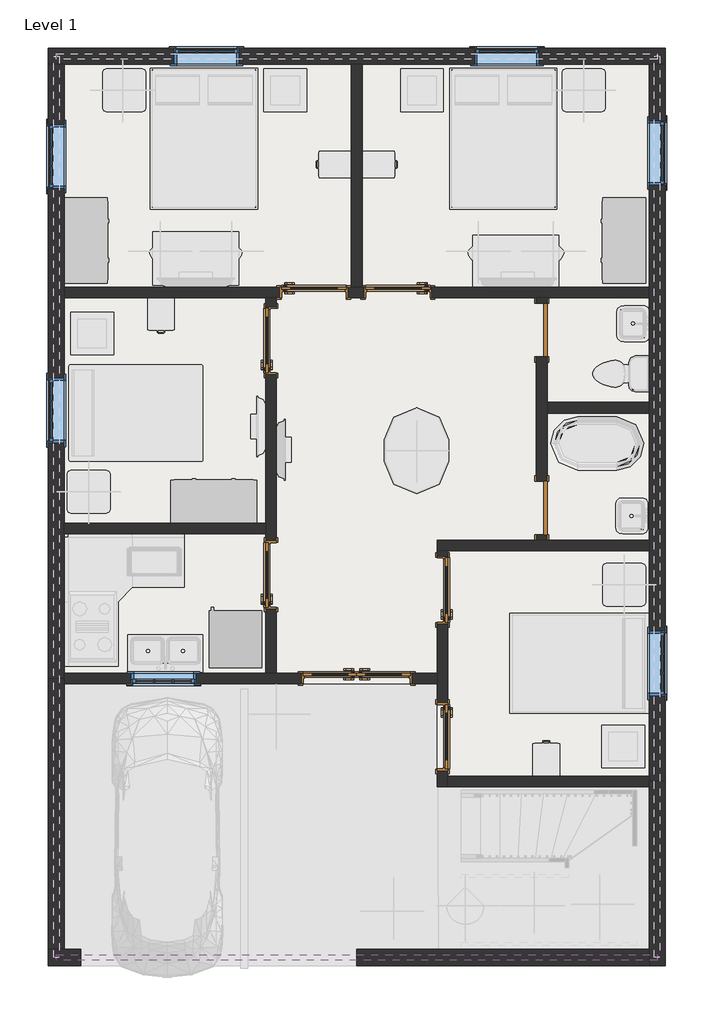
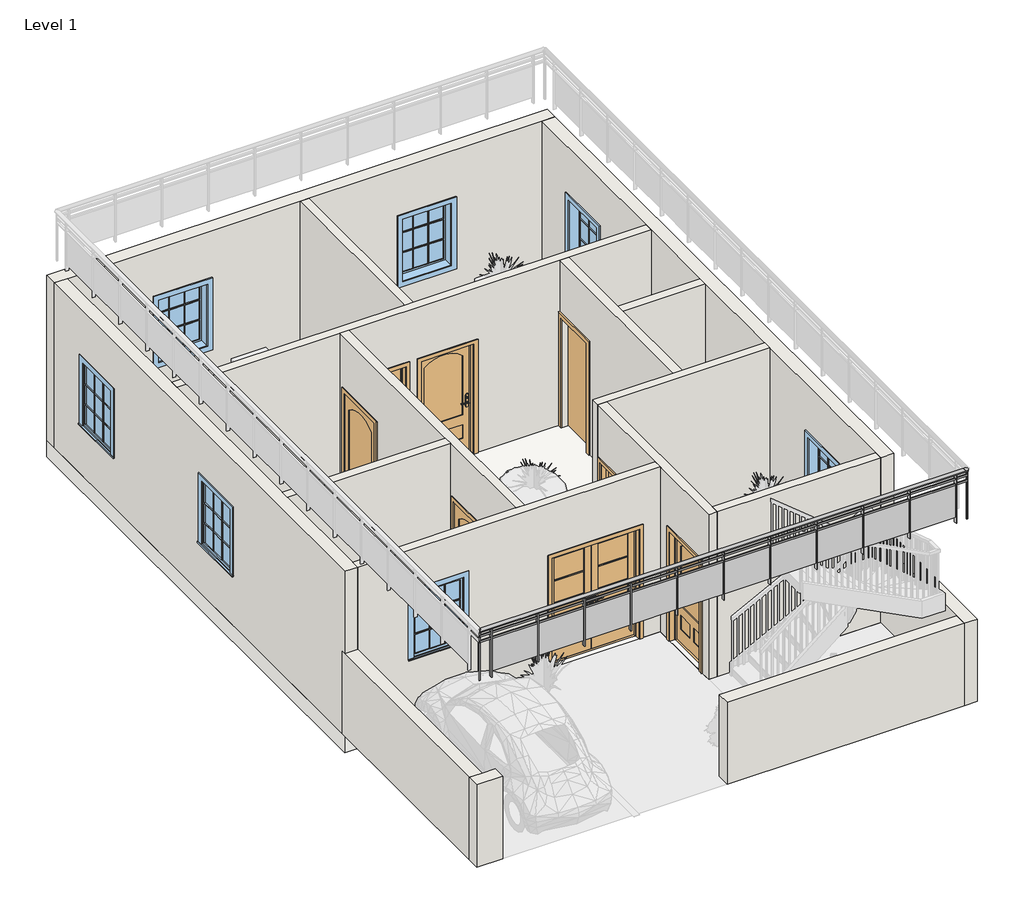
# One storey, part 1 of 4: 17 walls, 9 doors, 7 windows, 1 railing, 1 slab.
"""IFC4 building model written with IfcOpenShell, lengths in millimetres."""

from ifc_helpers import new_model, si_unit, point, frame, origin, origin_with_axes, place, context, project, spatial, polyline, ellipse_curve, trimmed, outline, extrude, faceted_brep, transform, mapped, element, save
from ifc_brep_helpers import plane_surface, extruded_surface, advanced_brep
from components import door_5d363d20, door_808aeb8e, door_94998e6c, door_255cab33, door_059fdd7e, window_b7d400b3, window_5c190c7e

model = new_model("IFC4")

# Units and contexts
model_context = context("Model", 3, world=origin())
ifc_project = project(units=[si_unit("LENGTHUNIT", "METRE", prefix="MILLI")], contexts=[model_context])

# Site, building, storey
site = spatial("IfcSite", under=ifc_project)
building = spatial("IfcBuilding", under=site)
storey = spatial("IfcBuildingStorey", under=building, Name="Level 1", Elevation=0.0)

# Doors
placement = place(None, origin())
door_shape = door_5d363d20(model_context)
element("IfcDoor", 1, ObjectType="36\" x 80\"", at=placement, inside=storey, context=model_context, shape_type="MappedRepresentation", body=[
    mapped(door_shape, transform((-9076.3505662, 9737.6395941, 0.0), x_axis=(-1.0, 0.0, 0.0), y_axis=(0.0, -1.0, 0.0), z_axis=(0.0, 0.0, 1.0))),
])
element("IfcDoor", 2, ObjectType="36\" x 80\"", at=placement, inside=storey, context=model_context, shape_type="MappedRepresentation", body=[
    mapped(door_shape, transform((-9689.1255662, 9048.6645941, 0.0), x_axis=(0.0, -1.0, 0.0), y_axis=(1.0, 0.0, 0.0), z_axis=(0.0, 0.0, 1.0))),
])
element("IfcDoor", 3, ObjectType="36\" x 80\"", at=placement, inside=storey, context=model_context, shape_type="MappedRepresentation", body=[
    mapped(door_shape, transform((-9689.1255662, 5721.2645941, 0.0), x_axis=(0.0, -1.0, 0.0), y_axis=(1.0, 0.0, 0.0), z_axis=(0.0, 0.0, 1.0))),
])
element("IfcDoor", 4, ObjectType="36\" x 80\"", at=placement, inside=storey, context=model_context, shape_type="MappedRepresentation", body=[
    mapped(door_shape, transform((-7244.3755662, 3422.5645941, 0.0), x_axis=(0.0, 1.0, 0.0), y_axis=(-1.0, 0.0, 0.0), z_axis=(0.0, 0.0, 1.0))),
])
door_2_shape = door_808aeb8e(model_context)
element("IfcDoor", 5, ObjectType="36\" x 80\"", at=placement, inside=storey, context=model_context, shape_type="MappedRepresentation", body=[
    mapped(door_2_shape, transform((-7882.5505662, 9737.6395941, 0.0), x_axis=(1.0, 0.0, 0.0), y_axis=(0.0, 1.0, 0.0), z_axis=(0.0, 0.0, 1.0))),
])
element("IfcDoor", 6, ObjectType="36\" x 80\"", at=placement, inside=storey, context=model_context, shape_type="MappedRepresentation", body=[
    mapped(door_2_shape, transform((-7244.3755662, 5505.3645941, 0.0), x_axis=(0.0, -1.0, 0.0), y_axis=(1.0, 0.0, 0.0), z_axis=(0.0, 0.0, 1.0))),
])
door_3_shape = door_94998e6c(model_context)
element("IfcDoor", 7, ObjectType="Door-Exterior-Double-Full Glass-Wood_Clad : 60\" x 80\"", at=placement, inside=storey, context=model_context, shape_type="MappedRepresentation", body=[
    mapped(door_3_shape, transform((-8466.7505662, 4251.2395941, 0.0), x_axis=(1.0, 0.0, 0.0), y_axis=(0.0, 1.0, 0.0), z_axis=(0.0, 0.0, 1.0))),
])
door_4_shape = door_255cab33(model_context)
element("IfcDoor", 8, ObjectType="Single-Flush : 30\" x 80\"", at=placement, inside=storey, context=model_context, shape_type="MappedRepresentation", body=[
    mapped(door_4_shape, transform((-5837.8505662, 9201.0645941, 0.0), x_axis=(0.0, 1.0, 0.0), y_axis=(-1.0, 0.0, 0.0), z_axis=(0.0, 0.0, 1.0))),
])
door_5_shape = door_059fdd7e(model_context)
element("IfcDoor", 9, ObjectType="Single-Flush : 30\" x 80\"", at=placement, inside=storey, context=model_context, shape_type="MappedRepresentation", body=[
    mapped(door_5_shape, transform((-5837.8505662, 6673.7645941, 0.0), x_axis=(0.0, -1.0, 0.0), y_axis=(1.0, 0.0, 0.0), z_axis=(0.0, 0.0, 1.0))),
])

# Railing
element("IfcRailing", 10, ObjectType="Glass Panel - Bottom Fill", at=placement, inside=storey, context=model_context, shape_type="SolidModel", body=[
    advanced_brep(
    [(-4199.5505662, 247.5645941, 4267.2), (-4199.5505662, 323.7645941, 4267.2), (-12733.9505662, 247.5645941, 4267.2), (-12733.9505662, 323.7645941, 4267.2)],
    [
        (0, 1, ellipse_curve(frame((-4199.5505662, 285.6645941, 4267.2), z_axis=(1.0, 0.0, 0.0), x_axis=(0.0, 1.0, 0.0)), 38.1, 28.575)),
        (1, 0, ellipse_curve(frame((-4199.5505662, 285.6645941, 4267.2), z_axis=(1.0, 0.0, 0.0), x_axis=(0.0, 1.0, 0.0)), 38.1, 28.575)),
        (2, 3, ellipse_curve(frame((-12733.9505662, 285.6645941, 4267.2), z_axis=(-1.0, 0.0, 0.0), x_axis=(0.0, 1.0, 0.0)), 38.1, 28.575)),
        (3, 2, ellipse_curve(frame((-12733.9505662, 285.6645941, 4267.2), z_axis=(-1.0, 0.0, 0.0), x_axis=(0.0, 1.0, 0.0)), 38.1, 28.575)),
        (0, 2),
        (3, 1),
    ],
    [
        plane_surface(frame((-4199.5505662, 285.6645941, 4267.2), z_axis=(1.0, 0.0, 0.0), x_axis=(0.0, -1.0, 0.0))),
        plane_surface(frame((-12733.9505662, 285.6645941, 4267.2), z_axis=(-1.0, 0.0, 0.0), x_axis=(0.0, -1.0, 0.0))),
        extruded_surface(trimmed(ellipse_curve(frame((-12733.9505662, 285.6645941, 4267.2), z_axis=(1.0, 0.0, 0.0), x_axis=(0.0, 1.0, 0.0)), 38.1, 28.575), [point((-12733.9505662, 247.5645941, 4267.2))], [point((-12733.9505662, 323.7645941, 4267.2))], True, "CARTESIAN"), (8534.4, 0.0, 0.0), 8534.4),
        extruded_surface(trimmed(ellipse_curve(frame((-12733.9505662, 285.6645941, 4267.2), z_axis=(1.0, 0.0, 0.0), x_axis=(0.0, 1.0, 0.0)), 38.1, 28.575), [point((-12733.9505662, 323.7645941, 4267.2))], [point((-12733.9505662, 247.5645941, 4267.2))], True, "CARTESIAN"), (8534.4, 0.0, 0.0), 8534.4),
    ],
    [
        (0, [[1, 2]]),
        (1, [[3, 4]]),
        (2, [[-1, 5, -4, 6]]),
        (3, [[-2, -6, -3, -5]]),
    ],
),
    extrude(outline(polyline([(-4199.5505662, 298.3645941), (-4199.5505662, 272.9645941), (-12733.9505662, 272.9645941), (-12733.9505662, 298.3645941), (-4199.5505662, 298.3645941)])), frame((0.0, 0.0, 4152.9), z_axis=(0.0, 0.0, 1.0), x_axis=(1.0, 0.0, 0.0)), (0.0, 0.0, 1.0), 25.4),
    extrude(outline(polyline([(-4199.5505662, 298.3645941), (-4199.5505662, 272.9645941), (-12733.9505662, 272.9645941), (-12733.9505662, 298.3645941), (-4199.5505662, 298.3645941)])), frame((0.0, 0.0, 4051.3), z_axis=(0.0, 0.0, 1.0), x_axis=(1.0, 0.0, 0.0)), (0.0, 0.0, 1.0), 25.4),
    extrude(outline(polyline([(-12524.4005662, 311.0645941), (-12524.4005662, 260.2645941), (-12537.1005662, 260.2645941), (-12537.1005662, 311.0645941), (-12524.4005662, 311.0645941)])), frame((0.0, 0.0, 3352.8), z_axis=(0.0, 0.0, 1.0), x_axis=(1.0, 0.0, 0.0)), (0.0, 0.0, 1.0), 885.6788223),
    extrude(outline(polyline([(-11717.9505662, 279.1294371), (-12530.7505662, 279.1294371), (-12530.7505662, 285.4794371), (-11717.9505662, 285.4794371), (-11717.9505662, 279.1294371)])), frame((0.0, 0.0, 3454.4), z_axis=(0.0, 0.0, 1.0), x_axis=(1.0, 0.0, 0.0)), (0.0, 0.0, 1.0), 596.9),
    extrude(outline(polyline([(-11711.6005662, 311.0645941), (-11711.6005662, 260.2645941), (-11724.3005662, 260.2645941), (-11724.3005662, 311.0645941), (-11711.6005662, 311.0645941)])), frame((0.0, 0.0, 3352.8), z_axis=(0.0, 0.0, 1.0), x_axis=(1.0, 0.0, 0.0)), (0.0, 0.0, 1.0), 885.6788223),
    extrude(outline(polyline([(-10905.1505662, 279.1294371), (-11717.9505662, 279.1294371), (-11717.9505662, 285.4794371), (-10905.1505662, 285.4794371), (-10905.1505662, 279.1294371)])), frame((0.0, 0.0, 3454.4), z_axis=(0.0, 0.0, 1.0), x_axis=(1.0, 0.0, 0.0)), (0.0, 0.0, 1.0), 596.9),
    extrude(outline(polyline([(-10898.8005662, 311.0645941), (-10898.8005662, 260.2645941), (-10911.5005662, 260.2645941), (-10911.5005662, 311.0645941), (-10898.8005662, 311.0645941)])), frame((0.0, 0.0, 3352.8), z_axis=(0.0, 0.0, 1.0), x_axis=(1.0, 0.0, 0.0)), (0.0, 0.0, 1.0), 885.6788223),
    extrude(outline(polyline([(-10092.3505662, 279.1294371), (-10905.1505662, 279.1294371), (-10905.1505662, 285.4794371), (-10092.3505662, 285.4794371), (-10092.3505662, 279.1294371)])), frame((0.0, 0.0, 3454.4), z_axis=(0.0, 0.0, 1.0), x_axis=(1.0, 0.0, 0.0)), (0.0, 0.0, 1.0), 596.9),
    extrude(outline(polyline([(-10086.0005662, 311.0645941), (-10086.0005662, 260.2645941), (-10098.7005662, 260.2645941), (-10098.7005662, 311.0645941), (-10086.0005662, 311.0645941)])), frame((0.0, 0.0, 3352.8), z_axis=(0.0, 0.0, 1.0), x_axis=(1.0, 0.0, 0.0)), (0.0, 0.0, 1.0), 885.6788223),
    extrude(outline(polyline([(-9279.5505662, 279.1294371), (-10092.3505662, 279.1294371), (-10092.3505662, 285.4794371), (-9279.5505662, 285.4794371), (-9279.5505662, 279.1294371)])), frame((0.0, 0.0, 3454.4), z_axis=(0.0, 0.0, 1.0), x_axis=(1.0, 0.0, 0.0)), (0.0, 0.0, 1.0), 596.9),
    extrude(outline(polyline([(-9273.2005662, 311.0645941), (-9273.2005662, 260.2645941), (-9285.9005662, 260.2645941), (-9285.9005662, 311.0645941), (-9273.2005662, 311.0645941)])), frame((0.0, 0.0, 3352.8), z_axis=(0.0, 0.0, 1.0), x_axis=(1.0, 0.0, 0.0)), (0.0, 0.0, 1.0), 885.6788223),
    extrude(outline(polyline([(-8466.7505662, 279.1294371), (-9279.5505662, 279.1294371), (-9279.5505662, 285.4794371), (-8466.7505662, 285.4794371), (-8466.7505662, 279.1294371)])), frame((0.0, 0.0, 3454.4), z_axis=(0.0, 0.0, 1.0), x_axis=(1.0, 0.0, 0.0)), (0.0, 0.0, 1.0), 596.9),
    extrude(outline(polyline([(-8460.4005662, 311.0645941), (-8460.4005662, 260.2645941), (-8473.1005662, 260.2645941), (-8473.1005662, 311.0645941), (-8460.4005662, 311.0645941)])), frame((0.0, 0.0, 3352.8), z_axis=(0.0, 0.0, 1.0), x_axis=(1.0, 0.0, 0.0)), (0.0, 0.0, 1.0), 885.6788223),
    extrude(outline(polyline([(-7653.9505662, 279.1294371), (-8466.7505662, 279.1294371), (-8466.7505662, 285.4794371), (-7653.9505662, 285.4794371), (-7653.9505662, 279.1294371)])), frame((0.0, 0.0, 3454.4), z_axis=(0.0, 0.0, 1.0), x_axis=(1.0, 0.0, 0.0)), (0.0, 0.0, 1.0), 596.9),
    extrude(outline(polyline([(-7647.6005662, 311.0645941), (-7647.6005662, 260.2645941), (-7660.3005662, 260.2645941), (-7660.3005662, 311.0645941), (-7647.6005662, 311.0645941)])), frame((0.0, 0.0, 3352.8), z_axis=(0.0, 0.0, 1.0), x_axis=(1.0, 0.0, 0.0)), (0.0, 0.0, 1.0), 885.6788223),
    extrude(outline(polyline([(-6841.1505662, 279.1294371), (-7653.9505662, 279.1294371), (-7653.9505662, 285.4794371), (-6841.1505662, 285.4794371), (-6841.1505662, 279.1294371)])), frame((0.0, 0.0, 3454.4), z_axis=(0.0, 0.0, 1.0), x_axis=(1.0, 0.0, 0.0)), (0.0, 0.0, 1.0), 596.9),
    extrude(outline(polyline([(-6834.8005662, 311.0645941), (-6834.8005662, 260.2645941), (-6847.5005662, 260.2645941), (-6847.5005662, 311.0645941), (-6834.8005662, 311.0645941)])), frame((0.0, 0.0, 3352.8), z_axis=(0.0, 0.0, 1.0), x_axis=(1.0, 0.0, 0.0)), (0.0, 0.0, 1.0), 885.6788223),
    extrude(outline(polyline([(-6028.3505662, 279.1294371), (-6841.1505662, 279.1294371), (-6841.1505662, 285.4794371), (-6028.3505662, 285.4794371), (-6028.3505662, 279.1294371)])), frame((0.0, 0.0, 3454.4), z_axis=(0.0, 0.0, 1.0), x_axis=(1.0, 0.0, 0.0)), (0.0, 0.0, 1.0), 596.9),
    extrude(outline(polyline([(-6022.0005662, 311.0645941), (-6022.0005662, 260.2645941), (-6034.7005662, 260.2645941), (-6034.7005662, 311.0645941), (-6022.0005662, 311.0645941)])), frame((0.0, 0.0, 3352.8), z_axis=(0.0, 0.0, 1.0), x_axis=(1.0, 0.0, 0.0)), (0.0, 0.0, 1.0), 885.6788223),
    extrude(outline(polyline([(-5215.5505662, 279.1294371), (-6028.3505662, 279.1294371), (-6028.3505662, 285.4794371), (-5215.5505662, 285.4794371), (-5215.5505662, 279.1294371)])), frame((0.0, 0.0, 3454.4), z_axis=(0.0, 0.0, 1.0), x_axis=(1.0, 0.0, 0.0)), (0.0, 0.0, 1.0), 596.9),
    extrude(outline(polyline([(-5209.2005662, 311.0645941), (-5209.2005662, 260.2645941), (-5221.9005662, 260.2645941), (-5221.9005662, 311.0645941), (-5209.2005662, 311.0645941)])), frame((0.0, 0.0, 3352.8), z_axis=(0.0, 0.0, 1.0), x_axis=(1.0, 0.0, 0.0)), (0.0, 0.0, 1.0), 885.6788223),
    extrude(outline(polyline([(-4402.7505662, 279.1294371), (-5215.5505662, 279.1294371), (-5215.5505662, 285.4794371), (-4402.7505662, 285.4794371), (-4402.7505662, 279.1294371)])), frame((0.0, 0.0, 3454.4), z_axis=(0.0, 0.0, 1.0), x_axis=(1.0, 0.0, 0.0)), (0.0, 0.0, 1.0), 596.9),
    extrude(outline(polyline([(-4396.4005662, 311.0645941), (-4396.4005662, 260.2645941), (-4409.1005662, 260.2645941), (-4409.1005662, 311.0645941), (-4396.4005662, 311.0645941)])), frame((0.0, 0.0, 3352.8), z_axis=(0.0, 0.0, 1.0), x_axis=(1.0, 0.0, 0.0)), (0.0, 0.0, 1.0), 885.6788223),
    extrude(outline(polyline([(-12721.2505662, 295.1895941), (-12721.2505662, 276.1395941), (-12740.3005662, 276.1395941), (-12740.3005662, 295.1895941), (-12721.2505662, 295.1895941)])), frame((0.0, 0.0, 3352.8), z_axis=(0.0, 0.0, 1.0), x_axis=(1.0, 0.0, 0.0)), (0.0, 0.0, 1.0), 885.6788223),
    extrude(outline(polyline([(-4193.2005662, 295.1895941), (-4193.2005662, 276.1395941), (-4212.2505662, 276.1395941), (-4212.2505662, 295.1895941), (-4193.2005662, 295.1895941)])), frame((0.0, 0.0, 3352.8), z_axis=(0.0, 0.0, 1.0), x_axis=(1.0, 0.0, 0.0)), (0.0, 0.0, 1.0), 885.6788223),
])

# Slab
element("IfcSlab", 11, ObjectType="Generic - 12\"", at=placement, inside=storey, context=model_context, shape_type="SweptSolid", body=[
    extrude(outline(polyline([(-4085.2505662, 13201.5645941), (-4085.2505662, 2711.3645941), (-7323.7505662, 2711.3645941), (-7323.7505662, 4171.8645941), (-12848.2505662, 4171.8645941), (-12848.2505662, 13201.5645941), (-4085.2505662, 13201.5645941)])), frame((0.0, 0.0, -304.8), z_axis=(0.0, 0.0, 1.0), x_axis=(1.0, 0.0, 0.0)), (0.0, 0.0, 1.0), 304.8),
])

# Walls
element("IfcWall", 12, ObjectType="Generic - 8\"", at=placement, inside=storey, context=model_context, shape_type="Brep", body=[
    faceted_brep([(-12848.2505662, 12972.9645941, 0.0), (-12619.6505662, 12972.9645941, 0.0), (-8542.9505662, 12972.9645941, 0.0), (-8390.5505662, 12972.9645941, 0.0), (-4313.8505662, 12972.9645941, 0.0), (-4085.2505662, 12972.9645941, 0.0), (-4085.2505662, 12972.9645941, 3048.0), (-4313.8505662, 12972.9645941, 3048.0), (-8390.5505662, 12972.9645941, 3048.0), (-8542.9505662, 12972.9645941, 3048.0), (-12619.6505662, 12972.9645941, 3048.0), (-12848.2505662, 12972.9645941, 3048.0), (-10143.1505662, 12972.9645941, 2133.6), (-10143.1505662, 12972.9645941, 914.4), (-11057.5505662, 12972.9645941, 914.4), (-11057.5505662, 12972.9645941, 2133.6), (-5875.9505662, 12972.9645941, 2133.6), (-5875.9505662, 12972.9645941, 914.4), (-6790.3505662, 12972.9645941, 914.4), (-6790.3505662, 12972.9645941, 2133.6), (-12848.2505662, 13201.5645941, 0.0), (-12848.2505662, 13201.5645941, 3048.0), (-4085.2505662, 13201.5645941, 3048.0), (-4085.2505662, 13201.5645941, 0.0), (-10143.1505662, 13201.5645941, 2133.6), (-11057.5505662, 13201.5645941, 2133.6), (-11057.5505662, 13201.5645941, 914.4), (-10143.1505662, 13201.5645941, 914.4), (-5875.9505662, 13201.5645941, 2133.6), (-6790.3505662, 13201.5645941, 2133.6), (-6790.3505662, 13201.5645941, 914.4), (-5875.9505662, 13201.5645941, 914.4)], [[[0, 1, 2, 3, 4, 5, 6, 7, 8, 9, 10, 11], [12, 13, 14, 15], [16, 17, 18, 19]], [[20, 21, 22, 23], [24, 25, 26, 27], [28, 29, 30, 31]], [[5, 4, 3, 2, 1, 0, 20, 23]], [[6, 5, 23, 22]], [[0, 11, 21, 20]], [[13, 12, 24, 27]], [[14, 13, 27, 26]], [[15, 14, 26, 25]], [[12, 15, 25, 24]], [[17, 16, 28, 31]], [[18, 17, 31, 30]], [[19, 18, 30, 29]], [[16, 19, 29, 28]], [[11, 10, 9, 8, 7, 6, 22, 21]]]),
])
element("IfcWall", 13, ObjectType="Generic - 8\"", at=placement, inside=storey, context=model_context, shape_type="Brep", body=[
    faceted_brep([(-4313.8505662, 12972.9645941, 0.0), (-4313.8505662, 9810.6645941, 0.0), (-4313.8505662, 9658.2645941, 0.0), (-4313.8505662, 8172.3645941, 0.0), (-4313.8505662, 8019.9645941, 0.0), (-4313.8505662, 6216.5645941, 0.0), (-4313.8505662, 6064.1645941, 0.0), (-4313.8505662, 2863.7645941, 0.0), (-4313.8505662, 2787.5645941, 0.0), (-4313.8505662, 2787.5645941, 1524.0), (-4313.8505662, 2711.3645941, 1524.0), (-4313.8505662, 2711.3645941, 3048.0), (-4313.8505662, 2863.7645941, 3048.0), (-4313.8505662, 6064.1645941, 3048.0), (-4313.8505662, 6216.5645941, 3048.0), (-4313.8505662, 8019.9645941, 3048.0), (-4313.8505662, 8172.3645941, 3048.0), (-4313.8505662, 9658.2645941, 3048.0), (-4313.8505662, 9810.6645941, 3048.0), (-4313.8505662, 12972.9645941, 3048.0), (-4313.8505662, 11258.4645941, 2133.6), (-4313.8505662, 11258.4645941, 914.4), (-4313.8505662, 12172.8645941, 914.4), (-4313.8505662, 12172.8645941, 2133.6), (-4313.8505662, 4006.7645941, 2133.6), (-4313.8505662, 4006.7645941, 914.4), (-4313.8505662, 4921.1645941, 914.4), (-4313.8505662, 4921.1645941, 2133.6), (-4085.2505662, 12972.9645941, 0.0), (-4085.2505662, 12972.9645941, 3048.0), (-4085.2505662, 2711.3645941, 3048.0), (-4085.2505662, 2711.3645941, 1524.0), (-4085.2505662, 2787.5645941, 1524.0), (-4085.2505662, 2787.5645941, 0.0), (-4085.2505662, 11258.4645941, 2133.6), (-4085.2505662, 12172.8645941, 2133.6), (-4085.2505662, 12172.8645941, 914.4), (-4085.2505662, 11258.4645941, 914.4), (-4085.2505662, 4006.7645941, 2133.6), (-4085.2505662, 4921.1645941, 2133.6), (-4085.2505662, 4921.1645941, 914.4), (-4085.2505662, 4006.7645941, 914.4)], [[[0, 1, 2, 3, 4, 5, 6, 7, 8, 9, 10, 11, 12, 13, 14, 15, 16, 17, 18, 19], [20, 21, 22, 23], [24, 25, 26, 27]], [[28, 29, 30, 31, 32, 33], [34, 35, 36, 37], [38, 39, 40, 41]], [[8, 7, 6, 5, 4, 3, 2, 1, 0, 28, 33]], [[0, 19, 29, 28]], [[21, 20, 34, 37]], [[22, 21, 37, 36]], [[23, 22, 36, 35]], [[20, 23, 35, 34]], [[25, 24, 38, 41]], [[26, 25, 41, 40]], [[27, 26, 40, 39]], [[24, 27, 39, 38]], [[9, 8, 33, 32]], [[31, 10, 9, 32]], [[11, 10, 31, 30]], [[19, 18, 17, 16, 15, 14, 13, 12, 11, 30, 29]]]),
])
element("IfcWall", 14, ObjectType="Generic - 8\"", at=placement, inside=storey, context=model_context, shape_type="Brep", body=[
    faceted_brep([(-12619.6505662, 4248.0645941, 0.0), (-12619.6505662, 4324.2645941, 0.0), (-12619.6505662, 6305.4645941, 0.0), (-12619.6505662, 6457.8645941, 0.0), (-12619.6505662, 9658.2645941, 0.0), (-12619.6505662, 9810.6645941, 0.0), (-12619.6505662, 12972.9645941, 0.0), (-12619.6505662, 12972.9645941, 3048.0), (-12619.6505662, 9810.6645941, 3048.0), (-12619.6505662, 9658.2645941, 3048.0), (-12619.6505662, 6457.8645941, 3048.0), (-12619.6505662, 6305.4645941, 3048.0), (-12619.6505662, 4324.2645941, 3048.0), (-12619.6505662, 4171.8645941, 3048.0), (-12619.6505662, 4171.8645941, 1524.0), (-12619.6505662, 4248.0645941, 1524.0), (-12619.6505662, 8515.2645941, 2133.6), (-12619.6505662, 8515.2645941, 914.4), (-12619.6505662, 7600.8645941, 914.4), (-12619.6505662, 7600.8645941, 2133.6), (-12619.6505662, 12122.0645941, 2133.6), (-12619.6505662, 12122.0645941, 914.4), (-12619.6505662, 11207.6645941, 914.4), (-12619.6505662, 11207.6645941, 2133.6), (-12848.2505662, 4248.0645941, 0.0), (-12848.2505662, 4248.0645941, 1524.0), (-12848.2505662, 4171.8645941, 1524.0), (-12848.2505662, 4171.8645941, 3048.0), (-12848.2505662, 12972.9645941, 3048.0), (-12848.2505662, 12972.9645941, 0.0), (-12848.2505662, 8515.2645941, 2133.6), (-12848.2505662, 7600.8645941, 2133.6), (-12848.2505662, 7600.8645941, 914.4), (-12848.2505662, 8515.2645941, 914.4), (-12848.2505662, 12122.0645941, 2133.6), (-12848.2505662, 11207.6645941, 2133.6), (-12848.2505662, 11207.6645941, 914.4), (-12848.2505662, 12122.0645941, 914.4)], [[[0, 1, 2, 3, 4, 5, 6, 7, 8, 9, 10, 11, 12, 13, 14, 15], [16, 17, 18, 19], [20, 21, 22, 23]], [[24, 25, 26, 27, 28, 29], [30, 31, 32, 33], [34, 35, 36, 37]], [[6, 5, 4, 3, 2, 1, 0, 24, 29]], [[7, 6, 29, 28]], [[16, 19, 31, 30]], [[19, 18, 32, 31]], [[18, 17, 33, 32]], [[17, 16, 30, 33]], [[20, 23, 35, 34]], [[23, 22, 36, 35]], [[22, 21, 37, 36]], [[21, 20, 34, 37]], [[0, 15, 25, 24]], [[14, 26, 25, 15]], [[14, 13, 27, 26]], [[13, 12, 11, 10, 9, 8, 7, 28, 27]]]),
])
element("IfcWall", 15, ObjectType="INNER 6\"", at=placement, inside=storey, context=model_context, shape_type="SweptSolid", body=[
    extrude(outline(polyline([(-8542.9505662, 9810.6645941), (-8542.9505662, 12972.9645941), (-8390.5505662, 12972.9645941), (-8390.5505662, 9810.6645941), (-8542.9505662, 9810.6645941)])), origin_with_axes(), (0.0, 0.0, 1.0), 3048.0),
])
element("IfcWall", 16, ObjectType="INNER 6\"", at=placement, inside=storey, context=model_context, shape_type="Brep", body=[
    faceted_brep([(-12619.6505662, 9810.6645941, 0.0), (-12619.6505662, 9810.6645941, 3048.0), (-8542.9505662, 9810.6645941, 3048.0), (-8390.5505662, 9810.6645941, 3048.0), (-4313.8505662, 9810.6645941, 3048.0), (-4313.8505662, 9810.6645941, 0.0), (-7399.9505662, 9810.6645941, 0.0), (-7399.9505662, 9810.6645941, 2057.4), (-8365.1505662, 9810.6645941, 2057.4), (-8365.1505662, 9810.6645941, 0.0), (-8390.5505662, 9810.6645941, 0.0), (-8542.9505662, 9810.6645941, 0.0), (-8593.7505662, 9810.6645941, 0.0), (-8593.7505662, 9810.6645941, 2057.4), (-9558.9505662, 9810.6645941, 2057.4), (-9558.9505662, 9810.6645941, 0.0), (-12619.6505662, 9658.2645941, 3048.0), (-12619.6505662, 9658.2645941, 0.0), (-9762.1505662, 9658.2645941, 0.0), (-9609.7505662, 9658.2645941, 0.0), (-9558.9505662, 9658.2645941, 0.0), (-9558.9505662, 9658.2645941, 2057.4), (-8593.7505662, 9658.2645941, 2057.4), (-8593.7505662, 9658.2645941, 0.0), (-8365.1505662, 9658.2645941, 0.0), (-8365.1505662, 9658.2645941, 2057.4), (-7399.9505662, 9658.2645941, 2057.4), (-7399.9505662, 9658.2645941, 0.0), (-5914.0505662, 9658.2645941, 0.0), (-5761.6505662, 9658.2645941, 0.0), (-4313.8505662, 9658.2645941, 0.0), (-4313.8505662, 9658.2645941, 3048.0), (-5761.6505662, 9658.2645941, 3048.0), (-5914.0505662, 9658.2645941, 3048.0), (-9609.7505662, 9658.2645941, 3048.0), (-9762.1505662, 9658.2645941, 3048.0)], [[[0, 1, 2, 3, 4, 5, 6, 7, 8, 9, 10, 11, 12, 13, 14, 15]], [[16, 17, 18, 19, 20, 21, 22, 23, 24, 25, 26, 27, 28, 29, 30, 31, 32, 33, 34, 35]], [[17, 0, 15, 20, 19, 18]], [[5, 30, 29, 28, 27, 6]], [[23, 12, 11, 10, 9, 24]], [[1, 0, 17, 16]], [[5, 4, 31, 30]], [[14, 21, 20, 15]], [[21, 14, 13, 22]], [[22, 13, 12, 23]], [[26, 7, 6, 27]], [[7, 26, 25, 8]], [[8, 25, 24, 9]], [[4, 3, 2, 1, 16, 35, 34, 33, 32, 31]]]),
])
element("IfcWall", 17, ObjectType="INNER 6\"", at=placement, inside=storey, context=model_context, shape_type="Brep", body=[
    faceted_brep([(-9762.1505662, 9658.2645941, 3048.0), (-9762.1505662, 9658.2645941, 0.0), (-9762.1505662, 9531.2645941, 0.0), (-9762.1505662, 9531.2645941, 2057.4), (-9762.1505662, 8566.0645941, 2057.4), (-9762.1505662, 8566.0645941, 0.0), (-9762.1505662, 6457.8645941, 0.0), (-9762.1505662, 6305.4645941, 0.0), (-9762.1505662, 6203.8645941, 0.0), (-9762.1505662, 6203.8645941, 2057.4), (-9762.1505662, 5238.6645941, 2057.4), (-9762.1505662, 5238.6645941, 0.0), (-9762.1505662, 4324.2645941, 0.0), (-9762.1505662, 4324.2645941, 3048.0), (-9762.1505662, 6305.4645941, 3048.0), (-9762.1505662, 6457.8645941, 3048.0), (-9609.7505662, 9658.2645941, 0.0), (-9609.7505662, 9658.2645941, 3048.0), (-9609.7505662, 4324.2645941, 3048.0), (-9609.7505662, 4324.2645941, 0.0), (-9609.7505662, 5238.6645941, 0.0), (-9609.7505662, 5238.6645941, 2057.4), (-9609.7505662, 6203.8645941, 2057.4), (-9609.7505662, 6203.8645941, 0.0), (-9609.7505662, 8566.0645941, 0.0), (-9609.7505662, 8566.0645941, 2057.4), (-9609.7505662, 9531.2645941, 2057.4), (-9609.7505662, 9531.2645941, 0.0)], [[[0, 1, 2, 3, 4, 5, 6, 7, 8, 9, 10, 11, 12, 13, 14, 15]], [[16, 17, 18, 19, 20, 21, 22, 23, 24, 25, 26, 27]], [[1, 16, 27, 2]], [[5, 24, 23, 8, 7, 6]], [[19, 12, 11, 20]], [[1, 0, 17, 16]], [[13, 12, 19, 18]], [[4, 25, 24, 5]], [[25, 4, 3, 26]], [[26, 3, 2, 27]], [[10, 21, 20, 11]], [[21, 10, 9, 22]], [[22, 9, 8, 23]], [[0, 15, 14, 13, 18, 17]]]),
])
element("IfcWall", 18, ObjectType="INNER 6\"", at=placement, inside=storey, context=model_context, shape_type="SweptSolid", body=[
    extrude(outline(polyline([(-12619.6505662, 6457.8645941), (-9762.1505662, 6457.8645941), (-9762.1505662, 6305.4645941), (-12619.6505662, 6305.4645941), (-12619.6505662, 6457.8645941)])), origin_with_axes(), (0.0, 0.0, 1.0), 3048.0),
])
element("IfcWall", 19, ObjectType="INNER 6\"", at=placement, inside=storey, context=model_context, shape_type="Brep", body=[
    faceted_brep([(-7323.7505662, 4324.2645941, 3048.0), (-7323.7505662, 4324.2645941, 0.0), (-7679.3505662, 4324.2645941, 0.0), (-7679.3505662, 4324.2645941, 2057.4), (-9254.1505662, 4324.2645941, 2057.4), (-9254.1505662, 4324.2645941, 0.0), (-9609.7505662, 4324.2645941, 0.0), (-9762.1505662, 4324.2645941, 0.0), (-12619.6505662, 4324.2645941, 0.0), (-12619.6505662, 4324.2645941, 3048.0), (-9762.1505662, 4324.2645941, 3048.0), (-9609.7505662, 4324.2645941, 3048.0), (-11667.1505662, 4324.2645941, 2235.2), (-11667.1505662, 4324.2645941, 1016.0), (-10752.7505662, 4324.2645941, 1016.0), (-10752.7505662, 4324.2645941, 2235.2), (-7323.7505662, 4171.8645941, 0.0), (-7323.7505662, 4171.8645941, 3048.0), (-12619.6505662, 4171.8645941, 3048.0), (-12619.6505662, 4171.8645941, 1524.0), (-12619.6505662, 4171.8645941, 0.0), (-9254.1505662, 4171.8645941, 0.0), (-9254.1505662, 4171.8645941, 2057.4), (-7679.3505662, 4171.8645941, 2057.4), (-7679.3505662, 4171.8645941, 0.0), (-11667.1505662, 4171.8645941, 2235.2), (-10752.7505662, 4171.8645941, 2235.2), (-10752.7505662, 4171.8645941, 1016.0), (-11667.1505662, 4171.8645941, 1016.0), (-12619.6505662, 4248.0645941, 0.0)], [[[0, 1, 2, 3, 4, 5, 6, 7, 8, 9, 10, 11], [12, 13, 14, 15]], [[16, 17, 18, 19, 20, 21, 22, 23, 24], [25, 26, 27, 28]], [[1, 16, 24, 2]], [[20, 29, 8, 7, 6, 5, 21]], [[1, 0, 17, 16]], [[23, 3, 2, 24]], [[3, 23, 22, 4]], [[4, 22, 21, 5]], [[13, 12, 25, 28]], [[14, 13, 28, 27]], [[15, 14, 27, 26]], [[12, 15, 26, 25]], [[8, 29, 20, 19, 18, 9]], [[0, 11, 10, 9, 18, 17]]]),
])
element("IfcWall", 20, ObjectType="INNER 6\"", at=placement, inside=storey, context=model_context, shape_type="SweptSolid", body=[
    extrude(outline(polyline([(-4313.8505662, 8019.9645941), (-5761.6505662, 8019.9645941), (-5761.6505662, 8172.3645941), (-4313.8505662, 8172.3645941), (-4313.8505662, 8019.9645941)])), origin_with_axes(), (0.0, 0.0, 1.0), 3048.0),
])
element("IfcWall", 21, ObjectType="INNER 6\"", at=placement, inside=storey, context=model_context, shape_type="Brep", body=[
    faceted_brep([(-4313.8505662, 6216.5645941, 0.0), (-5761.6505662, 6216.5645941, 0.0), (-5914.0505662, 6216.5645941, 0.0), (-7323.7505662, 6216.5645941, 0.0), (-7323.7505662, 6216.5645941, 3048.0), (-5914.0505662, 6216.5645941, 3048.0), (-5761.6505662, 6216.5645941, 3048.0), (-4313.8505662, 6216.5645941, 3048.0), (-4313.8505662, 6064.1645941, 0.0), (-4313.8505662, 6064.1645941, 3048.0), (-7171.3505662, 6064.1645941, 3048.0), (-7323.7505662, 6064.1645941, 3048.0), (-7323.7505662, 6064.1645941, 0.0), (-7171.3505662, 6064.1645941, 0.0)], [[[0, 1, 2, 3, 4, 5, 6, 7]], [[8, 9, 10, 11, 12, 13]], [[3, 2, 1, 0, 8, 13, 12]], [[0, 7, 9, 8]], [[4, 3, 12, 11]], [[7, 6, 5, 4, 11, 10, 9]]]),
])
element("IfcWall", 22, ObjectType="INNER 6\"", at=placement, inside=storey, context=model_context, shape_type="Brep", body=[
    faceted_brep([(-5761.6505662, 6216.5645941, 0.0), (-5761.6505662, 6292.7645941, 0.0), (-5761.6505662, 6292.7645941, 2032.0), (-5761.6505662, 7054.7645941, 2032.0), (-5761.6505662, 7054.7645941, 0.0), (-5761.6505662, 8019.9645941, 0.0), (-5761.6505662, 8172.3645941, 0.0), (-5761.6505662, 8820.0645941, 0.0), (-5761.6505662, 8820.0645941, 2032.0), (-5761.6505662, 9582.0645941, 2032.0), (-5761.6505662, 9582.0645941, 0.0), (-5761.6505662, 9658.2645941, 0.0), (-5761.6505662, 9658.2645941, 3048.0), (-5761.6505662, 8172.3645941, 3048.0), (-5761.6505662, 8019.9645941, 3048.0), (-5761.6505662, 6216.5645941, 3048.0), (-5914.0505662, 6292.7645941, 2032.0), (-5914.0505662, 6292.7645941, 0.0), (-5914.0505662, 6216.5645941, 0.0), (-5914.0505662, 6216.5645941, 3048.0), (-5914.0505662, 9658.2645941, 3048.0), (-5914.0505662, 9658.2645941, 0.0), (-5914.0505662, 9582.0645941, 0.0), (-5914.0505662, 9582.0645941, 2032.0), (-5914.0505662, 8820.0645941, 2032.0), (-5914.0505662, 8820.0645941, 0.0), (-5914.0505662, 7054.7645941, 0.0), (-5914.0505662, 7054.7645941, 2032.0)], [[[0, 1, 2, 3, 4, 5, 6, 7, 8, 9, 10, 11, 12, 13, 14, 15]], [[16, 17, 18, 19, 20, 21, 22, 23, 24, 25, 26, 27]], [[11, 10, 22, 21]], [[26, 25, 7, 6, 5, 4]], [[18, 17, 1, 0]], [[0, 15, 19, 18]], [[12, 11, 21, 20]], [[23, 22, 10, 9]], [[24, 23, 9, 8]], [[25, 24, 8, 7]], [[2, 1, 17, 16]], [[3, 2, 16, 27]], [[4, 3, 27, 26]], [[15, 14, 13, 12, 20, 19]]]),
])
element("IfcWall", 23, ObjectType="INNER 6\"", at=placement, inside=storey, context=model_context, shape_type="Brep", body=[
    faceted_brep([(-7323.7505662, 6064.1645941, 3048.0), (-7323.7505662, 6064.1645941, 0.0), (-7323.7505662, 5987.9645941, 0.0), (-7323.7505662, 5987.9645941, 2057.4), (-7323.7505662, 5022.7645941, 2057.4), (-7323.7505662, 5022.7645941, 0.0), (-7323.7505662, 4324.2645941, 0.0), (-7323.7505662, 4171.8645941, 0.0), (-7323.7505662, 3905.1645941, 0.0), (-7323.7505662, 3905.1645941, 2057.4), (-7323.7505662, 2939.9645941, 2057.4), (-7323.7505662, 2939.9645941, 0.0), (-7323.7505662, 2711.3645941, 0.0), (-7323.7505662, 2711.3645941, 3048.0), (-7323.7505662, 4171.8645941, 3048.0), (-7323.7505662, 4324.2645941, 3048.0), (-7171.3505662, 6064.1645941, 0.0), (-7171.3505662, 6064.1645941, 3048.0), (-7171.3505662, 2863.7645941, 3048.0), (-7171.3505662, 2711.3645941, 3048.0), (-7171.3505662, 2711.3645941, 0.0), (-7171.3505662, 2863.7645941, 0.0), (-7171.3505662, 2939.9645941, 0.0), (-7171.3505662, 2939.9645941, 2057.4), (-7171.3505662, 3905.1645941, 2057.4), (-7171.3505662, 3905.1645941, 0.0), (-7171.3505662, 5022.7645941, 0.0), (-7171.3505662, 5022.7645941, 2057.4), (-7171.3505662, 5987.9645941, 2057.4), (-7171.3505662, 5987.9645941, 0.0)], [[[0, 1, 2, 3, 4, 5, 6, 7, 8, 9, 10, 11, 12, 13, 14, 15]], [[16, 17, 18, 19, 20, 21, 22, 23, 24, 25, 26, 27, 28, 29]], [[1, 16, 29, 2]], [[20, 12, 11, 22, 21]], [[5, 26, 25, 8, 7, 6]], [[1, 0, 17, 16]], [[13, 12, 20, 19]], [[4, 27, 26, 5]], [[27, 4, 3, 28]], [[28, 3, 2, 29]], [[24, 9, 8, 25]], [[9, 24, 23, 10]], [[10, 23, 22, 11]], [[0, 15, 14, 13, 19, 18, 17]]]),
])
element("IfcWall", 24, ObjectType="INNER 6\"", at=placement, inside=storey, context=model_context, shape_type="Brep", body=[
    faceted_brep([(-7171.3505662, 2711.3645941, 0.0), (-4313.8505662, 2711.3645941, 0.0), (-4313.8505662, 2711.3645941, 1524.0), (-4313.8505662, 2711.3645941, 3048.0), (-7171.3505662, 2711.3645941, 3048.0), (-7171.3505662, 2863.7645941, 0.0), (-7171.3505662, 2863.7645941, 3048.0), (-4313.8505662, 2863.7645941, 3048.0), (-4313.8505662, 2863.7645941, 0.0), (-4313.8505662, 2787.5645941, 0.0)], [[[0, 1, 2, 3, 4]], [[5, 6, 7, 8]], [[1, 0, 5, 8, 9]], [[0, 4, 6, 5]], [[1, 9, 8, 7, 3, 2]], [[4, 3, 7, 6]]]),
])
element("IfcWall", 25, ObjectType="OUTER 5'", at=placement, inside=storey, context=model_context, shape_type="SweptSolid", body=[
    extrude(outline(polyline([(-8466.7505662, 399.9645941), (-4313.8505662, 399.9645941), (-4313.8505662, 171.3645941), (-8466.7505662, 171.3645941), (-8466.7505662, 399.9645941)])), origin_with_axes(), (0.0, 0.0, 1.0), 1524.0),
])
element("IfcWall", 26, ObjectType="OUTER 5'", at=placement, inside=storey, context=model_context, shape_type="Brep", body=[
    faceted_brep([(-12619.6505662, 399.9645941, 0.0), (-12619.6505662, 4171.8645941, 0.0), (-12619.6505662, 4248.0645941, 0.0), (-12619.6505662, 4248.0645941, 1524.0), (-12619.6505662, 399.9645941, 1524.0), (-12848.2505662, 399.9645941, 0.0), (-12848.2505662, 399.9645941, 1524.0), (-12848.2505662, 4248.0645941, 1524.0), (-12848.2505662, 4248.0645941, 0.0)], [[[0, 1, 2, 3, 4]], [[5, 6, 7, 8]], [[2, 1, 0, 5, 8]], [[3, 2, 8, 7]], [[4, 3, 7, 6]], [[0, 4, 6, 5]]]),
])
element("IfcWall", 27, ObjectType="OUTER 5'", at=placement, inside=storey, context=model_context, shape_type="Brep", body=[
    faceted_brep([(-4313.8505662, 2787.5645941, 0.0), (-4313.8505662, 2711.3645941, 0.0), (-4313.8505662, 399.9645941, 0.0), (-4313.8505662, 171.3645941, 0.0), (-4313.8505662, 171.3645941, 1524.0), (-4313.8505662, 399.9645941, 1524.0), (-4313.8505662, 2787.5645941, 1524.0), (-4085.2505662, 2787.5645941, 0.0), (-4085.2505662, 2787.5645941, 1524.0), (-4085.2505662, 171.3645941, 1524.0), (-4085.2505662, 171.3645941, 0.0)], [[[0, 1, 2, 3, 4, 5, 6]], [[7, 8, 9, 10]], [[3, 2, 1, 0, 7, 10]], [[6, 5, 4, 9, 8]], [[0, 6, 8, 7]], [[4, 3, 10, 9]]]),
])
element("IfcWall", 28, ObjectType="OUTER 5'", at=placement, inside=storey, context=model_context, shape_type="Brep", body=[
    faceted_brep([(-12391.0505662, 399.9645941, 0.0), (-12619.6505662, 399.9645941, 0.0), (-12848.2505662, 399.9645941, 0.0), (-12848.2505662, 399.9645941, 1524.0), (-12619.6505662, 399.9645941, 1524.0), (-12391.0505662, 399.9645941, 1524.0), (-12391.0505662, 171.3645941, 0.0), (-12391.0505662, 171.3645941, 1524.0), (-12848.2505662, 171.3645941, 1524.0), (-12848.2505662, 171.3645941, 0.0)], [[[0, 1, 2, 3, 4, 5]], [[6, 7, 8, 9]], [[2, 1, 0, 6, 9]], [[5, 4, 3, 8, 7]], [[0, 5, 7, 6]], [[3, 2, 9, 8]]]),
])

# Windows
window_shape = window_b7d400b3(model_context)
element("IfcWindow", 29, ObjectType="Casement 3x3 with Trim : 36\" x 48\"", at=placement, inside=storey, context=model_context, shape_type="MappedRepresentation", body=[
    mapped(window_shape, transform((-10600.3505662, 13087.2645941, 0.0), x_axis=(1.0, 0.0, 0.0), y_axis=(0.0, 1.0, 0.0), z_axis=(0.0, 0.0, 1.0))),
])
element("IfcWindow", 30, ObjectType="Casement 3x3 with Trim : 36\" x 48\"", at=placement, inside=storey, context=model_context, shape_type="MappedRepresentation", body=[
    mapped(window_shape, transform((-6333.1505662, 13087.2645941, 0.0), x_axis=(1.0, 0.0, 0.0), y_axis=(0.0, 1.0, 0.0), z_axis=(0.0, 0.0, 1.0))),
])
element("IfcWindow", 31, ObjectType="Casement 3x3 with Trim : 36\" x 48\"", at=placement, inside=storey, context=model_context, shape_type="MappedRepresentation", body=[
    mapped(window_shape, transform((-4199.5505662, 11715.6645941, 0.0), x_axis=(0.0, -1.0, 0.0), y_axis=(1.0, 0.0, 0.0), z_axis=(0.0, 0.0, 1.0))),
])
element("IfcWindow", 32, ObjectType="Casement 3x3 with Trim : 36\" x 48\"", at=placement, inside=storey, context=model_context, shape_type="MappedRepresentation", body=[
    mapped(window_shape, transform((-4199.5505662, 4463.9645941, 0.0), x_axis=(0.0, -1.0, 0.0), y_axis=(1.0, 0.0, 0.0), z_axis=(0.0, 0.0, 1.0))),
])
element("IfcWindow", 33, ObjectType="Casement 3x3 with Trim : 36\" x 48\"", at=placement, inside=storey, context=model_context, shape_type="MappedRepresentation", body=[
    mapped(window_shape, transform((-12733.9505662, 8058.0645941, 0.0), x_axis=(0.0, 1.0, 0.0), y_axis=(-1.0, 0.0, 0.0), z_axis=(0.0, 0.0, 1.0))),
])
element("IfcWindow", 34, ObjectType="Casement 3x3 with Trim : 36\" x 48\"", at=placement, inside=storey, context=model_context, shape_type="MappedRepresentation", body=[
    mapped(window_shape, transform((-12733.9505662, 11664.8645941, 0.0), x_axis=(0.0, 1.0, 0.0), y_axis=(-1.0, 0.0, 0.0), z_axis=(0.0, 0.0, 1.0))),
])
window_2_shape = window_5c190c7e(model_context)
element("IfcWindow", 35, ObjectType="Casement 3x3 with Trim : 36\" x 48\"", at=placement, inside=storey, context=model_context, shape_type="MappedRepresentation", body=[
    mapped(window_2_shape, transform((-11209.9505662, 4248.0645941, 101.6), x_axis=(-1.0, 0.0, 0.0), y_axis=(0.0, -1.0, 0.0), z_axis=(0.0, 0.0, 1.0))),
])

save(model, "model.ifc")

# Revit data of these elements
# Type "36\" x 80\""
#   Type Mark = "8"
#   Assembly Code = "B2030100"
#   Analytic Construction = "French door, wood frame with single glass"
#   Threshold Offset [instance default] = 0' - 0 1/2"
#   Thickness = 0' - 1 3/8"
#   Thermal Resistance (R) = 1.0696 (h·ft²·°F)/BTU
#   Swing Angle [instance default] = 90.00°
#   Stiles = 0' - 4 3/4"
#   Rough Width = 3' - 2"
#   Rough Height = 6' - 9"
#   Radius = 1' - 8.05625"
#   Lock Rail = 0' - 7 1/8"
#   Height = 6' - 8"
#   Width = 3' - 0"
#   Heat Transfer Coefficient (U) = 0.9350 BTU/(h·ft²·°F)
#   Door Offset [instance default] = 0' - 0"
#   Bottom Rail = 0' - 9 1/2"
#   Threshold [instance default] = yes
#   Function = 1
#   Exterior Trim [instance default] = yes
#   Trim Material = Cherry
#   Threshold Material = Cherry
#   Panel Material = Cherry
#   Glazing = Glass
#   Frame Material = Cherry
#   Door Handle Material = Aluminum
#   Visual Light Transmittance = 0
#   Solar Heat Gain Coefficient = 0
#   Wall Closure = (empty or 0)
#   Construction Type = (empty or 0)
# Type "Door-Exterior-Double-Full Glass-Wood_Clad : 60\" x 80\""
#   Type Mark = "9"
#   Assembly Code = "B2030100"
#   Analytic Construction = "French door, wood frame with double glass"
#   Top Rail = 0' - 4 11/16"
#   Threshold Offset [instance default] = 0' - 0 1/2"
#   Thickness = 0' - 1 3/8"
#   Thermal Resistance (R) = 1.9158 (h·ft²·°F)/BTU
#   Swing Angle [instance default] = 90.00°
#   Stiles = 0' - 4 3/4"
#   Rough Width = 5' - 2"
#   Rough Height = 6' - 9"
#   Panel Width = 2' - 6"
#   Door Offset [instance default] = 0' - 0"
#   Height = 6' - 8"
#   Width = 5' - 0"
#   Heat Transfer Coefficient (U) = 0.5220 BTU/(h·ft²·°F)
#   Bottom Rail = 0' - 9 1/8"
#   Exterior Trim [instance default] = yes
#   Threshold [instance default] = yes
#   Show Grill [instance default] = yes
#   Function = 1
#   Trim Material = Cherry
#   Threshold Material = Cherry
#   Panel Material = Cherry
#   Glazing = Glass
#   Frame Material = Cherry
#   Door Handle Material = Aluminum
#   Visual Light Transmittance = 0
#   Solar Heat Gain Coefficient = 0
#   Wall Closure = (empty or 0)
#   Construction Type = (empty or 0)
# Type "Single-Flush : 30\" x 80\""
#   Type Mark = "5"
#   Construction Type Id = "MDOOR"
#   Assembly Code = "C1020"
#   Analytic Construction = "Metal"
#   Thickness = 0' - 2"
#   Heat Transfer Coefficient (U) = 0.651978 BTU/(h·ft²·°F)
#   Height = 6' - 8"
#   Trim Projection Ext = 0' - 1"
#   Trim Projection Int = 0' - 1"
#   Trim Width = 0' - 3"
#   Width = 2' - 6"
#   Define Thermal Properties by = 1
#   Door Material = Door - Panel
#   Frame Material = Door - Frame
#   Visual Light Transmittance = 0
#   Solar Heat Gain Coefficient = 0
#   Function = (empty or 0)
#   Wall Closure = (empty or 0)
# Type "Glass Panel - Bottom Fill"
#   Assembly Code = "C2010400"
#   built-in parameter 1008612 = 0.0416667 (stored number, unit not read)
#   built-in parameter 1008611 = 0.0416667 (stored number, unit not read)
#   built-in parameter 1008609 = 0.333333 (stored number, unit not read)
#   built-in parameter 1008604 = 0.166667 (stored number, unit not read)
#   built-in parameter 1008603 = 0.166667 (stored number, unit not read)
#   Railing Height = 3' - 0"
#   built-in parameter 1008630 = 2
#   built-in parameter 1008610 = 2
#   built-in parameter 1008618 = Baluster - Square : 3/4"
# Type "Generic - 12\""
#   Assembly Code = "B1010"
#   Function = 0
#   Layers, outside or top first: 1' - 0" no material (function 1)
# Type "Generic - 8\""
#   Assembly Code = "B2010"
#   Layers, outside or top first: 0' - 9" "Brick, Common" (function 1)
# Type "INNER 6\""
#   Assembly Code = "B2010"
#   Layers, outside or top first: 0' - 6" "Brick, Common" (function 1)
# Type "OUTER 5'"
#   Assembly Code = "B2010"
#   Layers, outside or top first: 0' - 9" "Birch" (function 1)
# Type "Casement 3x3 with Trim : 36\" x 48\""
#   Type Mark = "10"
#   Construction Type Id = "GSP4R"
#   Assembly Code = "B2020100"
#   Analytic Construction = "1/8 in Pilkington single glazing"
#   Visual Light Transmittance = 0.9
#   Solar Heat Gain Coefficient = 0.78
#   Heat Transfer Coefficient (U) = 0.6496 BTU/(h·ft²·°F)
#   Height = 4' - 0"
#   Default Sill Height = 3' - 0"
#   Trim Projection - Ext. = 0' - 0 1/2"
#   Trim Projection - Int. = 0' - 0 3/4"
#   Trim Width - Exterior = 0' - 3 1/2"
#   Trim Width - Interior = 0' - 3 1/2"
#   Width = 3' - 0"
#   Window Inset = 0' - 0 3/4"
#   Define Thermal Properties by = 1
#   Glass Pane Material = Glass
#   Sash Material = Sash
#   Trim Exterior Material = Trim
#   Trim Interior Material = Trim
#   Wall Closure = (empty or 0)
# Elements 1, 2, 3, 4, 5, 6 (IfcDoor, "36\" x 80\"")
#   Threshold Offset = 0' - 0 1/2"
#   Swing Angle = 90.00°
#   Door Offset = 0' - 0"
#   Threshold = yes
#   Exterior Trim = yes
#   Phase Created = New Construction
#   Materials on its faces: "Cherry", "Aluminum", "Glass"
# Element 7 (IfcDoor, "Door-Exterior-Double-Full Glass-Wood_Clad : 60\" x 80\"")
#   Threshold Offset = 0' - 0 1/2"
#   Swing Angle = 90.00°
#   Door Offset = 0' - 0"
#   Threshold = yes
#   Show Grill = yes
#   Exterior Trim = yes
#   Phase Created = New Construction
#   Materials on its faces: "Cherry", "Aluminum", "Glass"
# Elements 8, 9 (IfcDoor, "Single-Flush : 30\" x 80\"")
#   Phase Created = New Construction
#   Materials on its faces: "Door - Frame", "Door - Panel"
# Element 10 (IfcRailing, "Glass Panel - Bottom Fill")
#   built-in parameter 1008621 = 11 (stored number, unit not read)
#   Phase Created = New Construction
#   Materials on its faces: "Glass"
# Element 11 (IfcSlab, "Generic - 12\"")
#   Height Offset From Level = 0' - 0"
#   Phase Created = New Construction
#   Materials on its faces: "Default Floor"
# Elements 12, 13, 14 (IfcWall, "Generic - 8\"")
#   Top Offset = 0' - 0"
#   Base Offset = 0' - 0"
#   Unconnected Height = 10' - 0"
#   wall height = 10' - 0"
#   Phase Created = New Construction
#   Base Constraint = Level 1
#   Materials on its faces: "Brick, Common"
# Elements 15, 16, 17, 18, 19, 20, 21, 22, 23, 24 (IfcWall, "INNER 6\"")
#   Top Offset = 0' - 0"
#   Base Offset = 0' - 0"
#   Unconnected Height = 10' - 0"
#   wall height = 10' - 0"
#   Phase Created = New Construction
#   Base Constraint = Level 1
#   Materials on its faces: "Brick, Common"
# Elements 25, 26, 27, 28 (IfcWall, "OUTER 5'")
#   Top Offset = 0' - 0"
#   Base Offset = 0' - 0"
#   Unconnected Height = 5' - 0"
#   wall height = 5' - 0"
#   Phase Created = New Construction
#   Base Constraint = Level 1
#   Materials on its faces: "Birch"
# Element 29 (IfcWindow, "Casement 3x3 with Trim : 36\" x 48\"")
#   Mark = "1"
#   Phase Created = New Construction
#   Materials on its faces: "Sash", "Glass", "Trim"
# Element 30 (IfcWindow, "Casement 3x3 with Trim : 36\" x 48\"")
#   Mark = "2"
#   Phase Created = New Construction
#   Materials on its faces: "Sash", "Glass", "Trim"
# Element 31 (IfcWindow, "Casement 3x3 with Trim : 36\" x 48\"")
#   Mark = "3"
#   Phase Created = New Construction
#   Materials on its faces: "Sash", "Glass", "Trim"
# Element 32 (IfcWindow, "Casement 3x3 with Trim : 36\" x 48\"")
#   Mark = "4"
#   Phase Created = New Construction
#   Materials on its faces: "Sash", "Glass", "Trim"
# Element 33 (IfcWindow, "Casement 3x3 with Trim : 36\" x 48\"")
#   Mark = "6"
#   Phase Created = New Construction
#   Materials on its faces: "Sash", "Glass", "Trim"
# Element 34 (IfcWindow, "Casement 3x3 with Trim : 36\" x 48\"")
#   Mark = "7"
#   Phase Created = New Construction
#   Materials on its faces: "Sash", "Glass", "Trim"
# Element 35 (IfcWindow, "Casement 3x3 with Trim : 36\" x 48\"")
#   Mark = "5"
#   Phase Created = New Construction
#   Materials on its faces: "Sash", "Glass", "Trim"
# Materials
#   "Cherry": class "Wood", colour RGB 226 177 128, transparency 0, Description = "Prunus Serotina", Cost = 0
#   "Glass": class "Glass", colour RGB 0 128 192, transparency 0.75, Description = "Soda Lime Glass", Cost = 0
#   "Aluminum": class "Metal", colour RGB 247 247 247, transparency 0, Description = "Aluminum 6061", Cost = 0
#   "Door - Panel": class "Wood", colour RGB 210 159 95, transparency 0
#   "Door - Frame": colour RGB 118 70 51, transparency 0
#   "Brick, Common": class "Masonry", colour RGB 170 98 104, transparency 0, Description = "Common brick", Cost = 0
#   "Birch": class "Wood", colour RGB 224 178 126, transparency 0, Description = "Betula Alleghaniensis", Cost = 0
#   "Sash": class "Wood", colour RGB 224 178 126, transparency 0
#   "Trim": class "Wood", colour RGB 224 178 126, transparency 0
#   "Default Floor": colour RGB 128 128 128, transparency 0
# Room at (-10643.844, 11504.934) mm, phase "New Construction", upper level "Level 1", upper offset 10' - 0", lower offset 0' - 0"
#   Number = "1"
#   Name = "BEDROOM-1"
# Room at (-6428.857, 11212.987) mm, phase "New Construction", upper level "Level 1", upper offset 10' - 0", lower offset 0' - 0"
#   Number = "2"
#   Name = "BEDROOM-2"
# Room at (-11161.448, 7664.713) mm, phase "New Construction", upper level "Level 1", upper offset 10' - 0", lower offset 0' - 0"
#   Number = "3"
#   Name = "BEDROOM-3"
# Room at (-11218.715, 5175.009) mm, phase "New Construction", upper level "Level 1", upper offset 10' - 0", lower offset 0' - 0"
#   Number = "4"
#   Name = "KITCHEN"
# Room at (-4961.296, 8633.735) mm, phase "New Construction", upper level "Level 1", upper offset 10' - 0", lower offset 0' - 0"
#   Number = "5"
#   Name = "WC"
# Room at (-4961.296, 6936.689) mm, phase "New Construction", upper level "Level 1", upper offset 10' - 0", lower offset 0' - 0"
#   Number = "6"
#   Name = "BATH"
# Room at (-7899.676, 7664.713) mm, phase "New Construction", upper level "Level 1", upper offset 10' - 0", lower offset 0' - 0"
#   Number = "7"
#   Name = "HALL"
# Room at (-5546.413, 4359.757) mm, phase "New Construction", upper level "Level 1", upper offset 10' - 0", lower offset 0' - 0"
#   Number = "8"
#   Name = "GUEST ROOM"
# Room at (-11232.159, 2162.714) mm, phase "New Construction", upper level "Level 1", upper offset 10' - 0", lower offset 0' - 0"
#   Number = "9"
